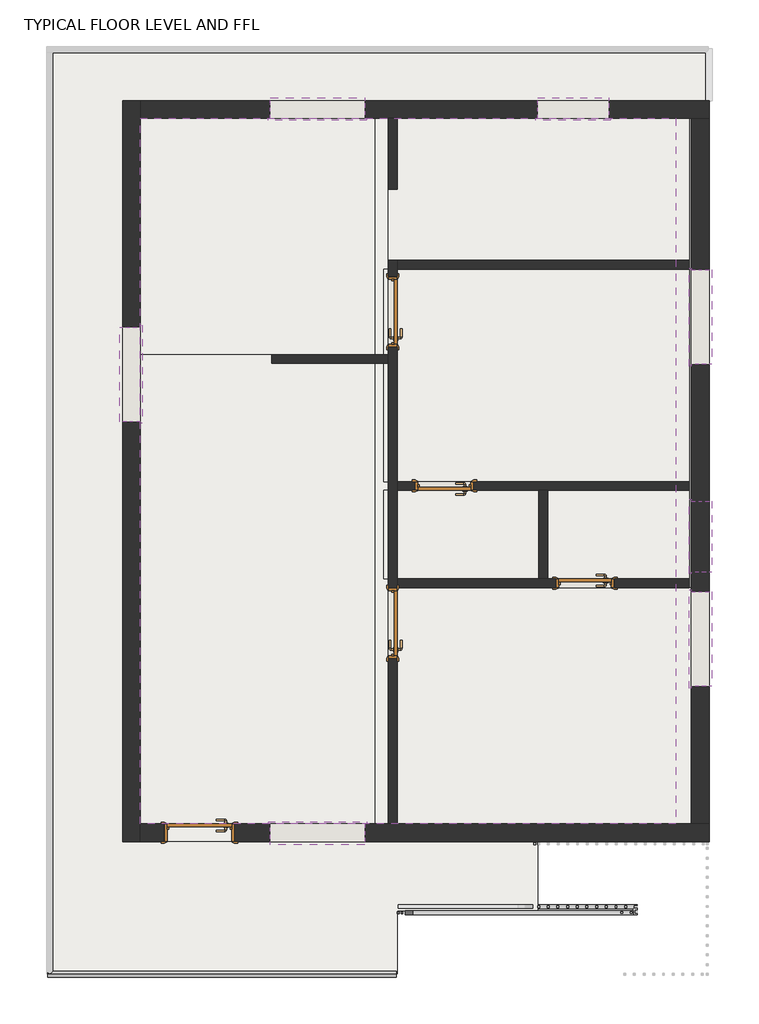
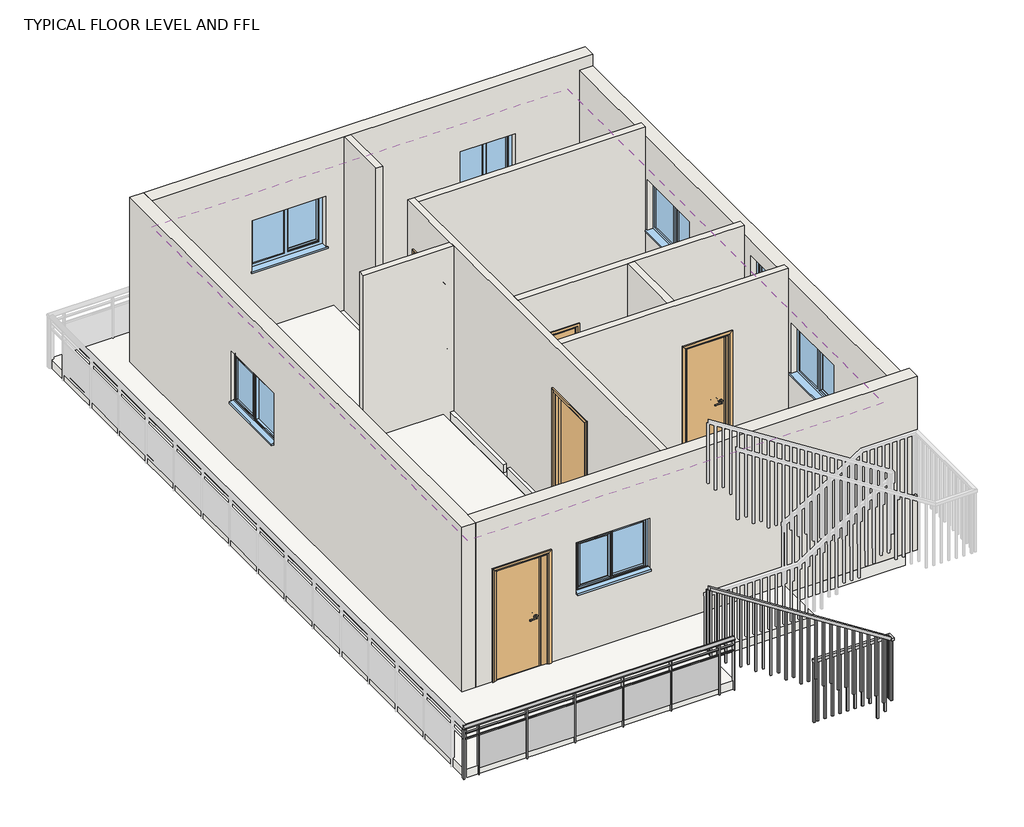
# One storey, part 1 of 3: 11 walls, 9 slabs, 7 windows, 5 doors, 2 railings, 1 covering.
# Revit data of these elements (continued)
# Elements 2, 3, 4 (IfcDoor, "Doors_IntSgl : D1") (continued)
#   Materials on its faces: "Door - Architrave", "Door - Handle", "Door - Frame/Mullion (1)", "Door - Panel"
# Elements 5, 6 (IfcDoor, "Doors_IntSgl : D2")
#   Phase Created = New Construction
#   Materials on its faces: "Door - Architrave", "Door - Handle", "Door - Frame/Mullion (1)", "Door - Panel"
# Element 7 (IfcRailing, "1100mm")
#   Phase Created = New Construction
# Element 8 (IfcRailing, "Glass_Panel-Bottom_Fill")
#   Phase Created = New Construction
#   Materials on its faces: "Metal - Stainless Steel,Polished", "Glass"
# Elements 9, 10 (IfcSlab, "BATHROOM FLOORING")
#   Height Offset From Level = 0.492 ft
#   Phase Created = New Construction
#   Materials on its faces: "Structure, Timber Joist/Rafter Layer", "BATHROOM FLOOR"
# Elements 11, 12 (IfcSlab, "BED ROOM FLOORING")
#   Height Offset From Level = 0.492 ft
#   Phase Created = New Construction
#   Materials on its faces: "Structure, Timber Joist/Rafter Layer", "BEDROOM FLOOR"
# Element 13 (IfcSlab, "DINING FLOORING")
#   Height Offset From Level = 0.492 ft
#   Phase Created = New Construction
#   Materials on its faces: "Structure, Timber Joist/Rafter Layer", "KITCHEN FLOOR"
# Element 14 (IfcSlab, "HALL FLOORING")
#   Height Offset From Level = 0.492 ft
#   Phase Created = New Construction
#   Materials on its faces: "Structure, Timber Joist/Rafter Layer", "HALL FLOOR"
# Element 15 (IfcSlab, "KITCHEN FLOOR")
#   Height Offset From Level = 0.492 ft
#   Phase Created = New Construction
#   Materials on its faces: "Structure, Timber Joist/Rafter Layer", "KITCHEN FLOOR"
# Element 16 (IfcSlab, "OUTER FLOORING")
#   Height Offset From Level = 0.492 ft
#   Phase Created = New Construction
#   Materials on its faces: "Structure, Timber Joist/Rafter Layer", "Concrete Masonry Units _High Density"
# Element 17 (IfcSlab, "RCC SLAB")
#   Height Offset From Level = 0.0 ft
#   built-in parameter 1001954 = 1
#   Phase Created = New Construction
# Elements 18, 19, 20 (IfcWall, "EXT WALL")
#   Top Offset = 0.0 ft
#   Base Offset = 0.0 ft
#   wall height = 10.0 ft
#   Phase Created = New Construction
#   Base Constraint = TYPICAL FLOOR LEVEL AND FFL
#   Top Constraint = SFL
#   Materials on its faces: "Brick, Common"
# Element 21 (IfcWall, "EXT WALL")
#   Top Offset = -0.656 ft
#   Base Offset = 0.0 ft
#   wall height = 9.344 ft
#   Phase Created = New Construction
#   Base Constraint = TYPICAL FLOOR LEVEL AND FFL
#   Top Constraint = SFL
#   Materials on its faces: "Brick, Common"
# Elements 22, 23, 24, 26, 27, 28 (IfcWall, "INT WALL")
#   Top Offset = 0.0 ft
#   Base Offset = 0.0 ft
#   wall height = 10.0 ft
#   Phase Created = New Construction
#   Base Constraint = TYPICAL FLOOR LEVEL AND FFL
#   Top Constraint = SFL
#   Materials on its faces: "Brick, Common"
# Element 25 (IfcWall, "INT WALL")
#   built-in parameter 1001111 = 0.010937 ft
#   Top Offset = 0.0 ft
#   Base Offset = 0.010937 ft
#   wall height = 9.989063 ft
#   Phase Created = New Construction
#   Base Constraint = TYPICAL FLOOR LEVEL AND FFL
#   Top Constraint = SFL
#   Materials on its faces: "Brick, Common"
# Elements 29, 30, 31, 32, 33 (IfcWindow, "Windows_Dbl_Plain : W1")
#   Mark = "W1"
#   Phase Created = New Construction
#   Materials on its faces: "Window Frame", "Glass"
# Element 34 (IfcWindow, "Windows_Dbl_Plain : W2")
#   Mark = "W2"
#   Phase Created = New Construction
#   Materials on its faces: "Window Frame", "Glass"
# Element 35 (IfcWindow, "Windows_Sgl_Plain : V")
#   Mark = "V"
#   Phase Created = New Construction
#   Materials on its faces: "Window Frame", "Glass"
# Materials
#   "Metal Stud Layer": class "Metal", colour RGB 127 127 127, transparency 0, Description = "Light gauge steel framing, thermal air layer", Cost = 0
#   "Gypsum Wall Board": class "Generic", colour RGB 249 249 249, transparency 0, Description = "Gypsum Wall Board", Cost = 0
#   "Door - Handle": colour RGB 0 0 0, transparency 0, Keynote = "P21", Cost = 0
#   "Door - Frame/Mullion (1)": class "Wood", colour RGB 212 179 113, transparency 0, Keynote = "L20", Cost = 0
#   "Door - Panel": class "Wood", colour RGB 210 159 95, transparency 0, Keynote = "L20", Cost = 0
#   "Door - Architrave": class "Wood", colour RGB 154 90 5, transparency 0, Keynote = "P20", Cost = 0
#   "BATHROOM FLOOR": class "Generic", colour RGB 120 120 120, transparency 0, Cost = 0
#   "Structure, Timber Joist/Rafter Layer": class "Wood", colour RGB 127 127 127, transparency 0, Description = "Timber framing, thermal airspace", Cost = 0
#   "BEDROOM FLOOR": class "Generic", colour RGB 120 120 120, transparency 0, Cost = 0
#   "KITCHEN FLOOR": class "Generic", colour RGB 120 120 120, transparency 0, Cost = 0
#   "HALL FLOOR": class "Generic", colour RGB 120 120 120, transparency 0, Cost = 0
#   "Concrete Masonry Units _High Density": class "Masonry", colour RGB 181 181 181, transparency 0, Description = "Concrete masonry units", Cost = 0
#   "Brick, Common": class "Masonry", colour RGB 170 100 105, transparency 0, Description = "Common brick", Cost = 0
#   "Window Frame": colour RGB 249 249 249, transparency 0, Keynote = "L10", Cost = 0
#   "Glass": class "Glass", colour RGB 0 128 192, transparency 0.9, Description = "Soda Lime Glass", Cost = 0
#   "Metal - Stainless Steel,Polished": class "Metal", colour RGB 236 239 239, transparency 0, Cost = 0
